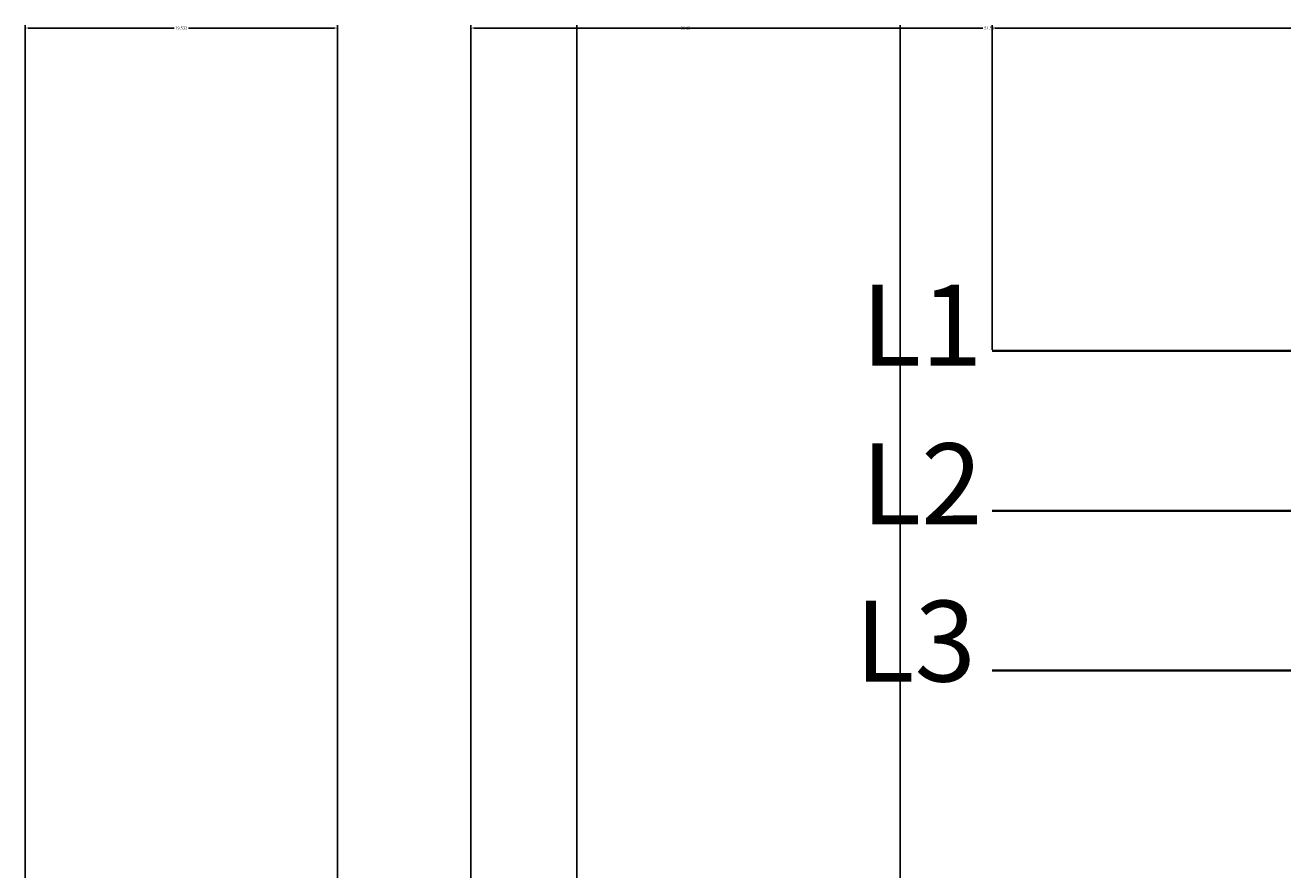
# Model space of a CAD drawing. Units: inches. Extents: x 738 to 1068, y 378 to 757.
# Tile 38 of 41: x 781 to 860, y 704 to 757. Entities that reach past the tile are written whole.
import ezdxf

# ---------------------------------------------------------------- set-up
doc = ezdxf.new("R2010")
doc.units = ezdxf.units.IN
doc.header["$MEASUREMENT"] = 0
for name, color, linetype, lineweight in [('A-ANNO-DIMS', 2, 'Continuous', 18), ('E-ANNO-TEXT', 7, 'Continuous', 18), ('E-POWR-FEED', 7, 'Continuous', 35)]:
    doc.layers.add(name, color=color, linetype=linetype, lineweight=lineweight)
doc.styles.get("Standard").update_dxf_attribs({"font": 'arial.ttf'})
doc.dimstyles.get("Standard").update_dxf_attribs({"dimtxt": 0.18, "dimasz": 0.18, "dimexe": 0.18, "dimexo": 0.0625, "dimgap": 0.09, "dimtad": 0, "dimtih": 1, "dimtoh": 1, "dimdec": 4, "dimzin": 0, "dimdsep": 46, "dimtxsty": 'Standard', "dimcen": 0.09, "dimadec": 0, "dimazin": 0, "dimtfac": 1, "dimtdec": 4, "dimtofl": 0, "dimtmove": 0, "dimatfit": 3, "dimfxl": 1, "dimtolj": 1, "dimtzin": 0, "dimarcsym": 0})

# ---------------------------------------------------------------- blocks, each defined once
blk = doc.blocks.new('*D26')
at = {"layer": 'A-ANNO-DIMS', "color": 0, "lineweight": -2, "transparency": 16777216}
for p, q in [((816.008, 647.048), (816.008, 756.505)), ((816.188, 756.325), (841.408, 756.325)), ((867.416, 756.325), (842.196, 756.325)), ((867.596, 647.048), (867.596, 756.505))]:
    blk.add_line(p, q, dxfattribs=at)
at = {"layer": 'A-ANNO-DIMS', "color": 0, "transparency": 16777216}
for points in [[(816.188, 756.355), (816.188, 756.295), (816.008, 756.325)], [(867.416, 756.355), (867.416, 756.295), (867.596, 756.325)]]:
    blk.add_solid(points, dxfattribs=at)
at = {"layer": 'Defpoints', "color": 0, "transparency": 16777216}
for p in [(867.596, 756.325), (816.008, 646.985), (867.596, 646.985)]:
    blk.add_point(p, dxfattribs=at)
at = {"layer": 'A-ANNO-DIMS', "color": 0, "transparency": 16777216, "insert": (841.802, 756.325), "char_height": 0.18, "attachment_point": 5}
blk.add_mtext('\\A1;51.59', dxfattribs=at)
blk = doc.blocks.new('*D31')
at = {"layer": 'A-ANNO-DIMS', "color": 0, "lineweight": -2, "transparency": 16777216}
for p, q in [((781.49, 531.463), (781.49, 756.505)), ((781.67, 756.325), (790.802, 756.325)), ((800.842, 756.325), (791.71, 756.325)), ((801.022, 531.463), (801.022, 756.505))]:
    blk.add_line(p, q, dxfattribs=at)
at = {"layer": 'A-ANNO-DIMS', "color": 0, "transparency": 16777216}
for points in [[(781.67, 756.355), (781.67, 756.295), (781.49, 756.325)], [(800.842, 756.355), (800.842, 756.295), (801.022, 756.325)]]:
    blk.add_solid(points, dxfattribs=at)
at = {"layer": 'Defpoints', "color": 0, "transparency": 16777216}
for p in [(801.022, 756.325), (781.49, 531.401), (801.022, 531.401)]:
    blk.add_point(p, dxfattribs=at)
at = {"layer": 'A-ANNO-DIMS', "color": 0, "transparency": 16777216, "insert": (791.256, 756.325), "char_height": 0.18, "attachment_point": 5}
blk.add_mtext('\\A1;19.532', dxfattribs=at)
blk = doc.blocks.new('*D32')
at = {"layer": 'A-ANNO-DIMS', "color": 0, "lineweight": -2, "transparency": 16777216}
for p, q in [((809.38, 461.454), (809.38, 756.505)), ((809.56, 756.325), (822.41, 756.325)), ((836.052, 756.325), (823.202, 756.325)), ((836.232, 461.277), (836.232, 756.505))]:
    blk.add_line(p, q, dxfattribs=at)
at = {"layer": 'A-ANNO-DIMS', "color": 0, "transparency": 16777216}
for points in [[(809.56, 756.355), (809.56, 756.295), (809.38, 756.325)], [(836.052, 756.355), (836.052, 756.295), (836.232, 756.325)]]:
    blk.add_solid(points, dxfattribs=at)
at = {"layer": 'Defpoints', "color": 0, "transparency": 16777216}
for p in [(836.232, 756.325), (809.38, 461.392), (836.232, 461.214)]:
    blk.add_point(p, dxfattribs=at)
at = {"layer": 'A-ANNO-DIMS', "color": 0, "transparency": 16777216, "insert": (822.806, 756.325), "char_height": 0.18, "attachment_point": 5}
blk.add_mtext('\\A1;26.85', dxfattribs=at)
blk = doc.blocks.new('*D37')
at = {"layer": 'A-ANNO-DIMS', "color": 0, "lineweight": -2, "transparency": 16777216}
for p, q in [((841.982, 736.191), (841.982, 756.505)), ((842.162, 756.325), (871.328, 756.325)), ((901.282, 756.325), (872.116, 756.325)), ((901.462, 735.938), (901.462, 756.505))]:
    blk.add_line(p, q, dxfattribs=at)
at = {"layer": 'A-ANNO-DIMS', "color": 0, "transparency": 16777216}
for points in [[(842.162, 756.355), (842.162, 756.295), (841.982, 756.325)], [(901.282, 756.355), (901.282, 756.295), (901.462, 756.325)]]:
    blk.add_solid(points, dxfattribs=at)
at = {"layer": 'Defpoints', "color": 0, "transparency": 16777216}
for p in [(901.462, 756.325), (841.982, 736.128), (901.462, 735.875)]:
    blk.add_point(p, dxfattribs=at)
at = {"layer": 'A-ANNO-DIMS', "color": 0, "transparency": 16777216, "insert": (871.722, 756.325), "char_height": 0.18, "attachment_point": 5}
blk.add_mtext('\\A1;59.48', dxfattribs=at)

msp = doc.modelspace()

# ---------------------------------------------------------------- linework, layer by layer
at = {"layer": 'E-POWR-FEED'}
for p, q in [((841.9816, 736.1282), (1012.7462, 736.1282)), ((841.9816, 726.1282), (1012.7462, 726.1282)), ((841.9816, 716.1282), (1012.7462, 716.1282))]:
    msp.add_line(p, q, dxfattribs=at)

# ---------------------------------------------------------------- texts
at = {"layer": 'E-ANNO-TEXT'}
for s, p in [('L1', (833.795, 735.2057)), ('L2', (833.795, 725.2838)), (' L3', (831.844, 715.4382))]:
    msp.add_text(s, height=5.05994, dxfattribs=at).set_placement(p)

# ---------------------------------------------------------------- dimensions: what is measured, and where the dimension line sits
at = {"layer": 'A-ANNO-DIMS'}
for base, p1, p2, override, picture, middle in [((801.0218, 756.3251), (781.4897, 531.4009), (801.0218, 531.4009), {"dimdec": 3, "dimlfac": 1, "dimrnd": 0, "dimzin": 0, "dimdsep": 46, "dimlunit": 2}, '*D31', (791.2557, 756.3251)), ((836.2324, 756.3251), (809.3803, 461.3919), (836.2324, 461.214), {"dimdec": 2, "dimlfac": 1, "dimrnd": 0, "dimzin": 0, "dimdsep": 46, "dimlunit": 2}, '*D32', (822.8064, 756.3251)), ((867.5964, 756.3251), (816.0076, 646.9853), (867.5964, 646.9853), {"dimdec": 2, "dimlfac": 1, "dimrnd": 0, "dimzin": 0, "dimdsep": 46, "dimlunit": 2}, '*D26', (841.802, 756.3251)), ((901.4622, 756.3251), (841.9816, 736.1282), (901.4622, 735.8751), {"dimdec": 2, "dimlfac": 1, "dimrnd": 0, "dimzin": 0, "dimdsep": 46, "dimlunit": 2}, '*D37', (871.7219, 756.3251))]:
    dim = msp.add_linear_dim(base=base, p1=p1, p2=p2, dimstyle='Standard', override=override, dxfattribs=at)
    dim.commit()
    dim.dimension.update_dxf_attribs({"geometry": picture, "text_midpoint": middle})

doc.saveas('drawing.dxf')
